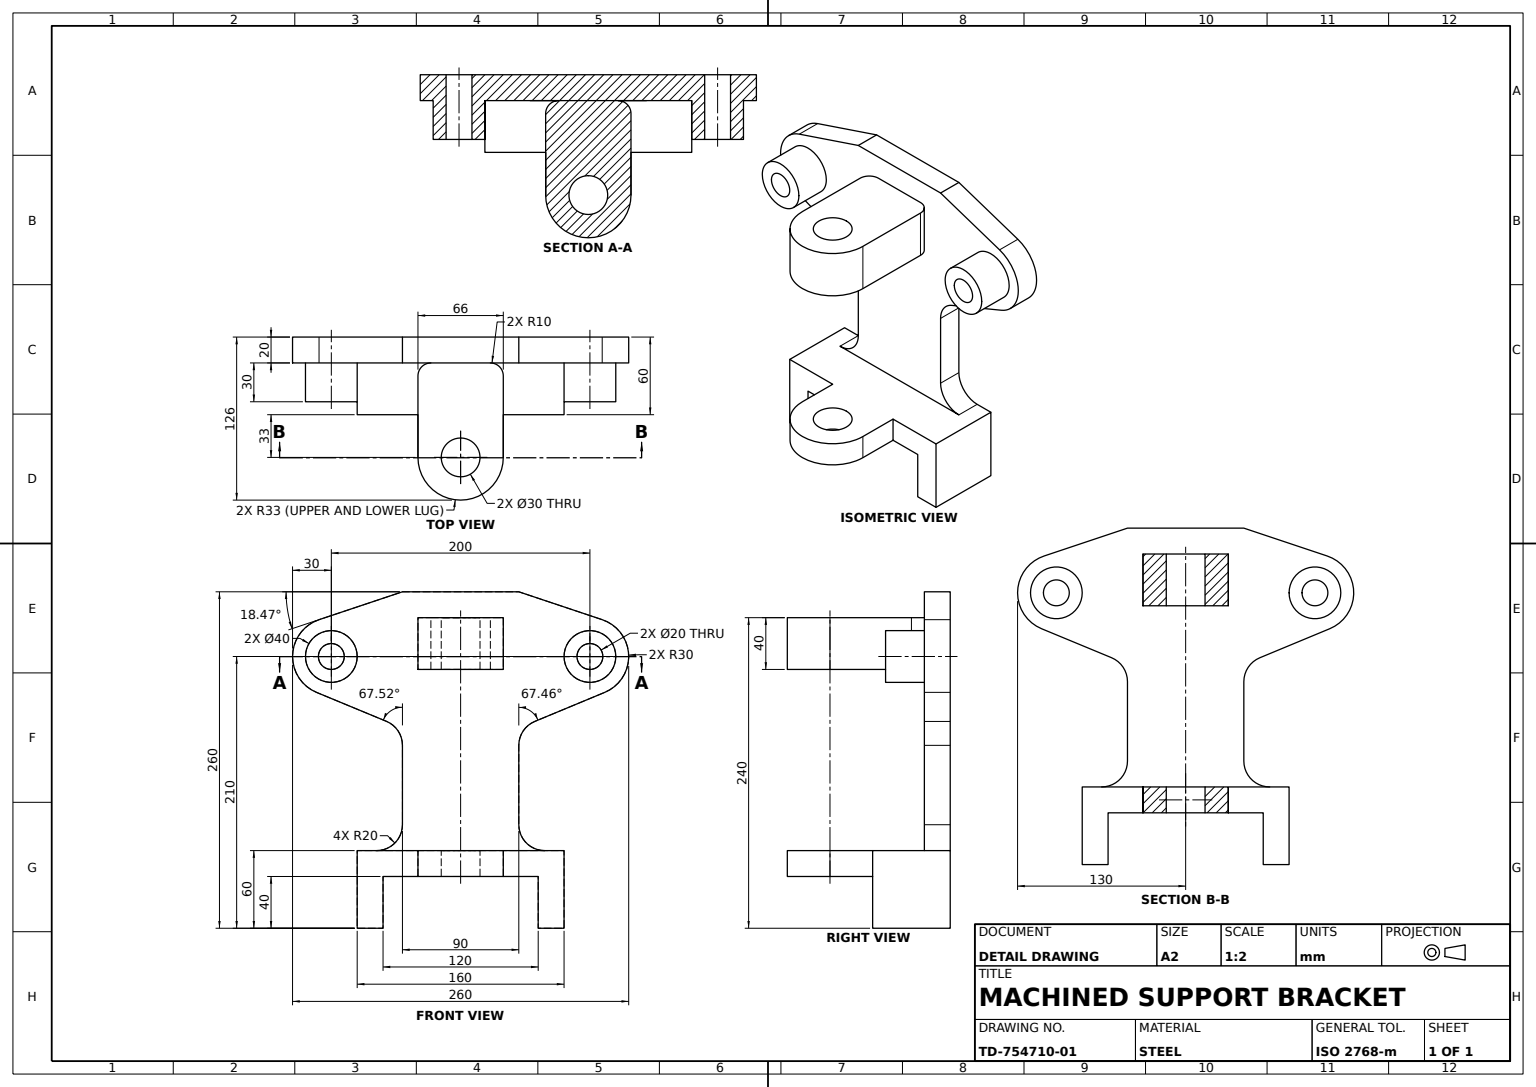
SolidWorks part; units mm, degrees
material "Plain Carbon Steel"
ref_plane "Front Plane" through (0, 0, 0) normal (0, 0, 1) x (1, 0, 0)
ref_plane "Top Plane" through (0, 0, 0) normal (0, 1, 0) x (1, 0, 0)
ref_plane "Right Plane" through (0, 0, 0) normal (1, 0, 0) x (0, 0, -1)
sketch "Base Web Sketch" plane through (0, 0, 0) normal (0, 0, 1) x (1, 0, 0)
  line L0 (0, 0) -> (0, 60)
  line L1 (0, 60) -> (160, 60)
  line L2 (160, 60) -> (160, 0)
  line L3 (160, 0) -> (140, 0)
  line L4 (140, 0) -> (140, 40)
  line L5 (140, 40) -> (20, 40)
  line L6 (20, 40) -> (20, 0)
  line L7 (20, 0) -> (0, 0)
  dimension "D1" = 60
  dimension "D2" = 160
  dimension "D3" = 120
  dimension "D4" = 20
  dimension "D5" = 40
extrude "Base Web" add sketch "Base Web Sketch" along normal blind 60
ref_plane "Upper Lug Plane" through (0, 60, 0) normal (0, 1, 0) x (1, 0, 0)
sketch "Upper Lug Sketch" plane through (0, 60, 0) normal (0, 1, 0) x (1, 0, 0)
  line L0 (80, -60) -> (80, -93) construction
  line L2 (160, -60) -> (0, -60) construction
  line L3 (47, -93) -> (47, -60)
  line L4 (113, -93) -> (113, -60)
  line L5 (47, -60) -> (113, -60)
  arc A1 (47, -93) -> (113, -93) centre (80, -93) ccw
  dimension "D1" = 66
  dimension "D2" = 33
extrude "Upper Lug" add sketch "Upper Lug Sketch" against normal blind 20
sketch "Upper Lug Bore Sketch" plane through (0, 60, 0) normal (0, 1, 0) x (1, 0, 0)
  circle A0 centre (80, -93) radius 15
  dimension "D1" = 30
extrude "Upper Lug Bore Ø30" cut sketch "Upper Lug Bore Sketch" against normal blind 20
ref_plane "Mounting Flange Plane" through (0, 0, 0) normal (0, 0, 1) x (1, 0, 0)
sketch "Mounting Flange Sketch" plane through (0, 0, 0) normal (0, 0, 1) x (1, 0, 0)
  line L0 (15, 60) -> (145, 60)
  line L1 (35, 260) -> (-29.5043, 238.4547)
  line L2 (125, 260) -> (189.5043, 238.4547)
  line L3 (-31.4702, 182.2794) -> (22.6468, 159.8868)
  line L4 (35, 260) -> (125, 260)
  line L5 (191.4994, 182.2914) -> (137.3338, 159.8121)
  line L6 (80, 210) -> (-20, 210) construction
  line L7 (80, 210) -> (180, 210) construction
  line L8 (35, 141.4064) -> (35, 80)
  line L9 (125, 141.3397) -> (125, 80)
  arc A0 (-29.5043, 238.4547) -> (-31.4702, 182.2794) centre (-20, 210) ccw
  arc A1 (191.4994, 182.2914) -> (189.5043, 238.4547) centre (180, 210) ccw
  arc A4 (15, 60) -> (35, 80) centre (15, 80) ccw
  arc A5 (125, 80) -> (145, 60) centre (145, 80) ccw
  arc A6 (125, 141.3397) -> (137.3338, 159.8121) centre (145, 141.3397) cw
  arc A7 (35, 141.4064) -> (22.6468, 159.8868) centre (15, 141.4064) ccw
  dimension "D2" = 60
  dimension "D3" = 60
  dimension "D12" = 40
  dimension "D13" = 40
  dimension "D14" = 60
  dimension "D11" = 20
  dimension "D6" = 210
  dimension "D7" = 180
  dimension "D8" = 20
  dimension "D9" = 64.5043
  dimension "D10" = 90
  dimension "D15" = 64.5043
  dimension "D16" = 54.1171
  dimension "D17" = 61.4064
  dimension "D18" = 54.1656
  dimension "D19" = 61.3397
extrude "Mounting Flange" add sketch "Mounting Flange Sketch" along normal blind 20
sketch "Flange Bosses Sketch" plane through (0, 0, 20) normal (0, 0, 1) x (1, 0, 0)
  circle A0 centre (-20, 210) radius 10
  circle A1 centre (-20, 210) radius 20
  circle A2 centre (180, 210) radius 10
  circle A3 centre (180, 210) radius 20
  dimension "D1" = 20
  dimension "D2" = 40
  dimension "D3" = 20
  dimension "D4" = 40
extrude "Flange Bosses" add sketch "Flange Bosses Sketch" along normal blind 30
ref_plane "Lower Lug Plane" through (0, 240, 0) normal (0, 1, 0) x (1, 0, 0)
sketch "Lower Lug Sketch" plane through (0, 240, 0) normal (0, 1, 0) x (1, 0, 0)
  line L2 (47, -93) -> (47, -30)
  line L3 (113, -93) -> (113, -30)
  line L5 (57, -20) -> (103, -20)
  circle A0 centre (80, -93) radius 15
  arc A1 (47, -93) -> (113, -93) centre (80, -93) ccw
  arc A2 (113, -30) -> (103, -20) centre (103, -30) ccw
  arc A3 (57, -20) -> (47, -30) centre (57, -30) ccw
  dimension "D1" = 30
  dimension "D3" = 10
  dimension "D2" = 20
extrude "Lower Lug" add sketch "Lower Lug Sketch" against normal blind 40
sketch "Flange Boss Holes Sketch" plane through (0, 0, 20) normal (0, 0, 1) x (1, 0, 0)
  circle A0 centre (-20, 210) radius 10
  circle A1 centre (180, 210) radius 10
  dimension "D1" = 20
extrude "Flange Boss Holes" cut sketch "Flange Boss Holes Sketch" against normal blind 40
